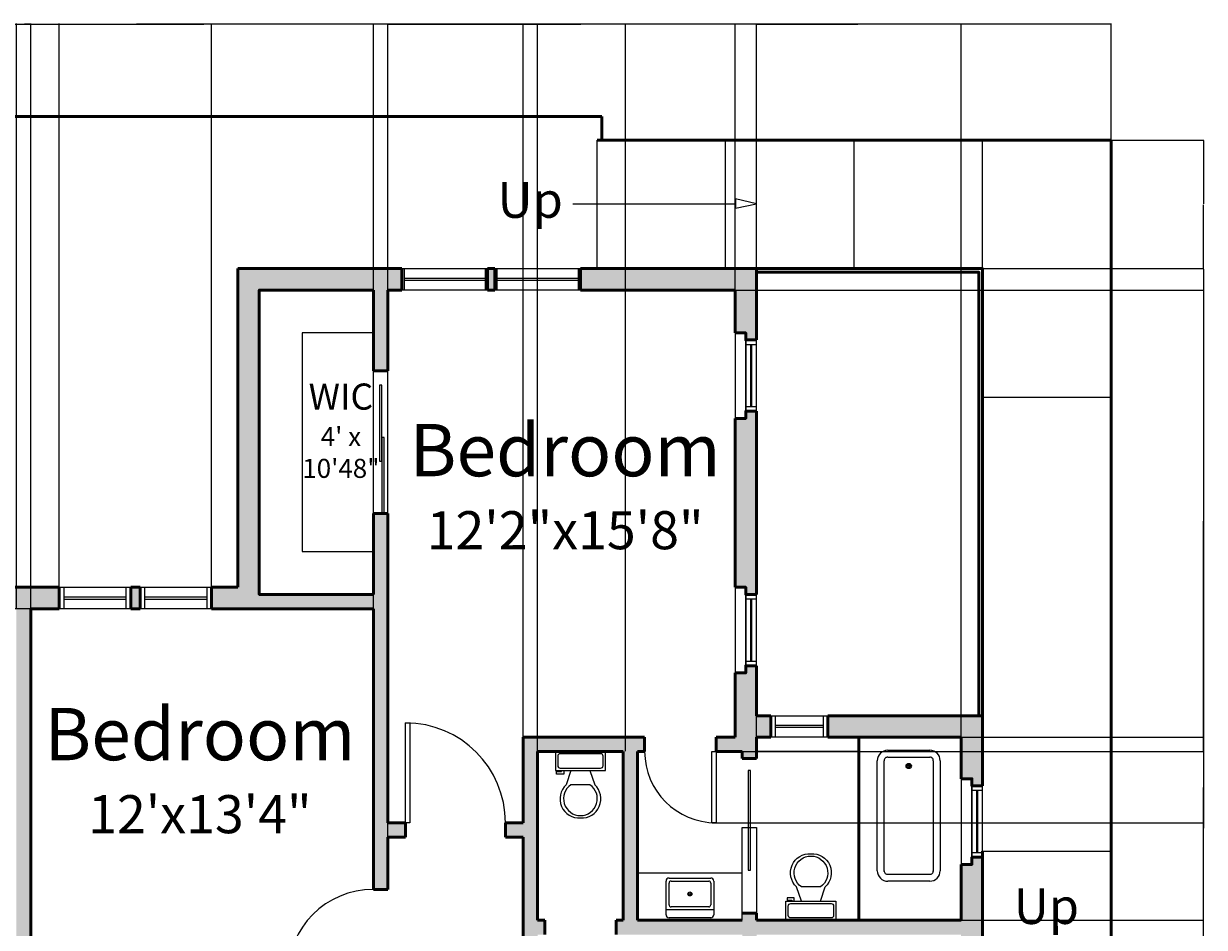
# Model space of a CAD drawing. Units: inches. Extents: x 296 to 2116, y 330 to 1460.
# Tile 9 of 9: x 1620 to 2116, y 1077 to 1457. Entities that reach past the tile are written whole.
import ezdxf

# ---------------------------------------------------------------- set-up
doc = ezdxf.new("R2010")
doc.units = ezdxf.units.IN
for name, color, linetype, lineweight in [('A-ANNO-DIMS', 2, 'Continuous', 18), ('A-ANNO-TEXT', 7, 'Continuous', 18), ('A-AREA-IDEN', 7, 'Continuous', 25), ('A-DOOR', 3, 'Continuous', 25), ('A-FLOR-FIXT', 8, 'Continuous', 18), ('A-FLOR-STRS', 40, 'Continuous', 25), ('A-GLAZ', 4, 'Continuous', 25), ('A-WALL', 7, 'Continuous', 50), ('A-WALL-PATT', 8, 'Continuous', 13)]:
    doc.layers.add(name, color=color, linetype=linetype, lineweight=lineweight)
doc.styles.add('ATTR', font='romans.shx', dxfattribs={"width": 0.8, "height": 1.075})
doc.styles.get("Standard").update_dxf_attribs({"font": 'arial.ttf'})
doc.dimstyles.get("Standard").update_dxf_attribs({"dimtxt": 0.18, "dimasz": 0.18, "dimexe": 0.18, "dimexo": 0.0625, "dimgap": 0.09, "dimtad": 0, "dimtih": 1, "dimtoh": 1, "dimdec": 4, "dimzin": 0, "dimdsep": 46, "dimtxsty": 'Standard', "dimcen": 0.09, "dimadec": 0, "dimazin": 0, "dimtfac": 1, "dimtdec": 4, "dimtofl": 0, "dimtmove": 0, "dimatfit": 3, "dimfxl": 1, "dimtolj": 1, "dimtzin": 0, "dimarcsym": 0})

# ---------------------------------------------------------------- blocks, each defined once
blk = doc.blocks.new('*U19')
for p, q in [((0, 0), (0, -4)), ((36, 0), (36, -4))]:
    blk.add_line(p, q)
blk.add_lwpolyline([(0, 0), (0, 36), (1.75, 36), (1.75, 0)], close=True)
blk.add_arc((0, 0), 36, 0, 90)
blk = doc.blocks.new('*U20')
for p, q in [((0, 0), (0, -4)), ((40, 0), (40, -4))]:
    blk.add_line(p, q)
blk.add_lwpolyline([(0, 0), (0, 40), (1.75, 40), (1.75, 0)], close=True)
blk.add_arc((0, 0), 40, 0, 90)
blk = doc.blocks.new('*U21')
for p, q in [((-30, 0), (-30, 4)), ((0, 0), (0, 4))]:
    blk.add_line(p, q)
blk.add_lwpolyline([(0, 0), (0, -30), (-1.75, -30), (-1.75, 0)], close=True)
blk.add_arc((0, 0), 30, 180, 270)
blk = doc.blocks.new('*U29')
for p, q in [((9.5, -6), (9.5, -2)), ((-10, -8.5), (-8, -8.5)), ((-10, -9.5), (-10, -8.5)), ((-7, -9.5), (-10, -9.5)), ((-8, -8.5), (-8, -8)), ((-7, -8), (-7, -9.5)), ((-4, -8), (-6, -14)), ((4, -8), (6, -14)), ((4, -14), (-4, -14))]:
    blk.add_line(p, q)
blk.add_lwpolyline([(10.5, -8), (10.5, 0), (-10.5, 0), (-10.5, -8)], close=True)
for points in [[(-9.5, -2), (-9.5, -6)], [(8.5, -1), (-8.5, -1)], [(-8.5, -7), (8.5, -7)]]:
    blk.add_lwpolyline(points)
for centre, radius, start, end in [((-8.625, -1.875), 0.8839, 81.8699, 188.1301), ((8.625, -1.875), 0.8839, 351.8699, 98.1301), ((-8.625, -6.125), 0.8839, 171.869898, 278.1301), ((8.625, -6.125), 0.8839, 261.8699, 8.1301), ((-0.4772, -19.9188), 8.0953, 133.01722, 273.38), ((0.0374, -19.8731), 7.127, 124.50543, 269.7), ((-0.0373, -19.8731), 7.127, 270.3, 55.4946), ((0.4773, -19.9188), 8.0953, 266.62, 46.9828)]:
    blk.add_arc(centre, radius, start, end)
blk = doc.blocks.new("24'' Sink Single PV")
blk.add_line((-12.00001, -3.999996), (12, -3.999996))
for points in [[(-10.5, 0), (10.5, 0)], [(-12.00001, -18.499996), (-12.00001, -1.5)], [(-9.5, -5.499996), (9.5, -5.499996)], [(12, -1.5), (12, -18.499996)], [(-10.5, -17.499996), (-10.5, -6.499996)], [(10.5, -6.499996), (10.5, -17.499996)], [(10.5, -19.999996), (-10.5, -19.999996)], [(9.5, -18.499996), (-9.5, -18.499996)]]:
    blk.add_lwpolyline(points)
for radius in [1, 0.5]:
    blk.add_circle((0, -11.999996), radius)
for centre, radius, start, end in [((-10.5, -1.5), 1.5, 90, 180), ((-9.5, -6.499996), 1, 90, 180), ((9.5, -6.499996), 1, 0, 90), ((10.5, -1.5), 1.5, 0, 90), ((-9.5, -17.499996), 1, 180, 270), ((9.5, -17.499996), 1, 270, 0), ((-10.5, -18.499996), 1.5, 180, 270), ((10.5, -18.499996), 1.5, 270, 0)]:
    blk.add_arc(centre, radius, start, end)
at = {"style": 'ATTR', "width": 0.8, "flags": 9}
blk.add_attdef('ESTCODE', (0, 0), '', height=0.0048, dxfattribs=at)
blk = doc.blocks.new('Bath Tub - 26 x 60 in.')
for p, q in [((6, 0), (69, 0)), ((0, -30), (0, -6)), ((75, -6), (75, -30)), ((8, -18), (10, -18)), ((9, -17), (9, -19)), ((69, -36), (6, -36))]:
    blk.add_line(p, q)
for points in [[(4, -30), (4, -6)], [(6, -4), (69.5, -4)], [(71, -30), (71, -6)], [(69.5, -32), (6, -32)]]:
    blk.add_lwpolyline(points)
for radius in [1.5, 1]:
    blk.add_circle((9, -18), radius)
for centre, radius, start, end in [((6, -6), 6, 90, 180), ((69, -6), 6, 0, 90), ((5.75, -5.75), 1.77, 81.8699, 188.1301), ((69.25, -5.75), 1.77, 351.8699, 98.1301), ((6, -30), 6, 180, 270), ((5.75, -30.25), 1.77, 171.8699, 278.1301), ((69.25, -30.25), 1.77, 261.8699, 8.1301), ((69, -30), 6, 270, 0)]:
    blk.add_arc(centre, radius, start, end)
blk = doc.blocks.new('*D67')
at = {"layer": 'A-ANNO-DIMS', "color": 0, "lineweight": -2, "transparency": 16777216}
for p, q in [((1315.18, 1418.02), (1315.18, 1456.98)), ((1315.36, 1456.8), (1695.9, 1456.8)), ((2077, 1456.8), (1696.47, 1456.8)), ((2077.18, 1408.02), (2077.18, 1456.98))]:
    blk.add_line(p, q, dxfattribs=at)
at = {"layer": 'A-ANNO-DIMS', "color": 0, "transparency": 16777216}
for points in [[(1315.36, 1456.83), (1315.36, 1456.77), (1315.18, 1456.8)], [(2077, 1456.83), (2077, 1456.77), (2077.18, 1456.8)]]:
    blk.add_solid(points, dxfattribs=at)
at = {"layer": 'Defpoints', "color": 0, "transparency": 16777216}
for p in [(2077.18, 1456.8), (1315.18, 1417.95), (2077.18, 1407.95)]:
    blk.add_point(p, dxfattribs=at)
at = {"layer": 'A-ANNO-DIMS', "color": 0, "transparency": 16777216, "insert": (1696.18, 1456.8), "char_height": 0.18, "attachment_point": 5}
blk.add_mtext('\\A1;762', dxfattribs=at)
blk = doc.blocks.new('*D74')
at = {"layer": 'A-ANNO-DIMS', "color": 0, "lineweight": -2, "transparency": 16777216}
for p, q in [((2023.25, 1353.95), (2116.21, 1353.95)), ((2116.03, 1353.77), (2116.03, 1129.14)), ((2116.03, 904.13), (2116.03, 1128.77)), ((2023.25, 903.95), (2116.21, 903.95))]:
    blk.add_line(p, q, dxfattribs=at)
at = {"layer": 'A-ANNO-DIMS', "color": 0, "transparency": 16777216}
for points in [[(2116, 1353.77), (2116.06, 1353.77), (2116.03, 1353.95)], [(2116, 904.13), (2116.06, 904.13), (2116.03, 903.95)]]:
    blk.add_solid(points, dxfattribs=at)
at = {"layer": 'Defpoints', "color": 0, "transparency": 16777216}
for p in [(2023.18, 1353.95), (2116.03, 1353.95), (2023.18, 903.95)]:
    blk.add_point(p, dxfattribs=at)
at = {"layer": 'A-ANNO-DIMS', "color": 0, "transparency": 16777216, "insert": (2116.03, 1128.95), "char_height": 0.18, "attachment_point": 5}
blk.add_mtext('\\A1;450', dxfattribs=at)
blk = doc.blocks.new('*D75')
at = {"layer": 'A-ANNO-DIMS', "color": 0, "lineweight": -2, "transparency": 16777216}
for p, q in [((2077.25, 1407.95), (2116.21, 1407.95)), ((2116.03, 1407.77), (2116.03, 1381.14)), ((2116.03, 1354.13), (2116.03, 1380.77)), ((2023.25, 1353.95), (2116.21, 1353.95))]:
    blk.add_line(p, q, dxfattribs=at)
at = {"layer": 'A-ANNO-DIMS', "color": 0, "transparency": 16777216}
for points in [[(2116, 1407.77), (2116.06, 1407.77), (2116.03, 1407.95)], [(2116, 1354.13), (2116.06, 1354.13), (2116.03, 1353.95)]]:
    blk.add_solid(points, dxfattribs=at)
at = {"layer": 'Defpoints', "color": 0, "transparency": 16777216}
for p in [(2077.18, 1407.95), (2116.03, 1407.95), (2023.18, 1353.95)]:
    blk.add_point(p, dxfattribs=at)
at = {"layer": 'A-ANNO-DIMS', "color": 0, "transparency": 16777216, "insert": (2116.03, 1380.95), "char_height": 0.18, "attachment_point": 5}
blk.add_mtext('\\A1;54', dxfattribs=at)
blk = doc.blocks.new('*D108')
at = {"layer": 'A-ANNO-DIMS', "color": 0, "lineweight": -2, "transparency": 16777216}
for p, q in [((1617.18, 1211.02), (1617.18, 1456.98)), ((1617.36, 1456.8), (1619.86, 1456.8)), ((1623, 1456.8), (1620.51, 1456.8)), ((1623.18, 1211.02), (1623.18, 1456.98))]:
    blk.add_line(p, q, dxfattribs=at)
at = {"layer": 'A-ANNO-DIMS', "color": 0, "transparency": 16777216}
for points in [[(1617.36, 1456.83), (1617.36, 1456.77), (1617.18, 1456.8)], [(1623, 1456.83), (1623, 1456.77), (1623.18, 1456.8)]]:
    blk.add_solid(points, dxfattribs=at)
at = {"layer": 'Defpoints', "color": 0, "transparency": 16777216}
for p in [(1623.18, 1456.8), (1617.18, 1210.95), (1623.18, 1210.95)]:
    blk.add_point(p, dxfattribs=at)
at = {"layer": 'A-ANNO-DIMS', "color": 0, "transparency": 16777216, "insert": (1620.18, 1456.8), "char_height": 0.18, "attachment_point": 5}
blk.add_mtext('\\A1;6.00', dxfattribs=at)
blk = doc.blocks.new('*D109')
at = {"layer": 'A-ANNO-DIMS', "color": 0, "lineweight": -2, "transparency": 16777216}
for p, q in [((1623.18, 1211.02), (1623.18, 1456.98)), ((1623.36, 1456.8), (1694.73, 1456.8)), ((1767, 1456.8), (1695.64, 1456.8)), ((1767.18, 1211.02), (1767.18, 1456.98))]:
    blk.add_line(p, q, dxfattribs=at)
at = {"layer": 'A-ANNO-DIMS', "color": 0, "transparency": 16777216}
for points in [[(1623.36, 1456.83), (1623.36, 1456.77), (1623.18, 1456.8)], [(1767, 1456.83), (1767, 1456.77), (1767.18, 1456.8)]]:
    blk.add_solid(points, dxfattribs=at)
at = {"layer": 'Defpoints', "color": 0, "transparency": 16777216}
for p in [(1767.18, 1456.8), (1623.18, 1210.95), (1767.18, 1210.95)]:
    blk.add_point(p, dxfattribs=at)
at = {"layer": 'A-ANNO-DIMS', "color": 0, "transparency": 16777216, "insert": (1695.18, 1456.8), "char_height": 0.18, "attachment_point": 5}
blk.add_mtext('\\A1;144.00', dxfattribs=at)
blk = doc.blocks.new('*D110')
at = {"layer": 'A-ANNO-DIMS', "color": 0, "lineweight": -2, "transparency": 16777216}
for p, q in [((1773.18, 1345.02), (1773.18, 1456.98)), ((1773.36, 1456.8), (1845.73, 1456.8)), ((1919, 1456.8), (1846.64, 1456.8)), ((1919.18, 1345.02), (1919.18, 1456.98))]:
    blk.add_line(p, q, dxfattribs=at)
at = {"layer": 'A-ANNO-DIMS', "color": 0, "transparency": 16777216}
for points in [[(1773.36, 1456.83), (1773.36, 1456.77), (1773.18, 1456.8)], [(1919, 1456.83), (1919, 1456.77), (1919.18, 1456.8)]]:
    blk.add_solid(points, dxfattribs=at)
at = {"layer": 'Defpoints', "color": 0, "transparency": 16777216}
for p in [(1919.18, 1456.8), (1773.18, 1344.95), (1919.18, 1344.95)]:
    blk.add_point(p, dxfattribs=at)
at = {"layer": 'A-ANNO-DIMS', "color": 0, "transparency": 16777216, "insert": (1846.18, 1456.8), "char_height": 0.18, "attachment_point": 5}
blk.add_mtext('\\A1;146.00', dxfattribs=at)
blk = doc.blocks.new('*D118')
at = {"layer": 'A-ANNO-DIMS', "color": 0, "lineweight": -2, "transparency": 16777216}
for p, q in [((1623.12, 1210.95), (1276.15, 1210.95)), ((1276.33, 1210.77), (1276.33, 1131.14)), ((1276.33, 1051.13), (1276.33, 1130.77)), ((1623.12, 1050.95), (1276.15, 1050.95))]:
    blk.add_line(p, q, dxfattribs=at)
at = {"layer": 'A-ANNO-DIMS', "color": 0, "transparency": 16777216}
for points in [[(1276.3, 1210.77), (1276.36, 1210.77), (1276.33, 1210.95)], [(1276.3, 1051.13), (1276.36, 1051.13), (1276.33, 1050.95)]]:
    blk.add_solid(points, dxfattribs=at)
at = {"layer": 'Defpoints', "color": 0, "transparency": 16777216}
for p in [(1276.33, 1210.95), (1623.18, 1210.95), (1623.18, 1050.95)]:
    blk.add_point(p, dxfattribs=at)
at = {"layer": 'A-ANNO-DIMS', "color": 0, "transparency": 16777216, "insert": (1276.33, 1130.95), "char_height": 0.18, "attachment_point": 5}
blk.add_mtext('\\A1;160.00', dxfattribs=at)
blk = doc.blocks.new('*D119')
at = {"layer": 'A-ANNO-DIMS', "color": 0, "lineweight": -2, "transparency": 16777216}
for p, q in [((1773.183215, 1093.016598), (1773.183215, 1456.984098)), ((1773.363215, 1456.804098), (1801.289818, 1456.804098)), ((1830.003215, 1456.804098), (1802.076612, 1456.804098)), ((1830.183215, 1157.016598), (1830.183215, 1456.984098))]:
    blk.add_line(p, q, dxfattribs=at)
at = {"layer": 'A-ANNO-DIMS', "color": 0, "transparency": 16777216}
for points in [[(1773.363215, 1456.834098), (1773.363215, 1456.774098), (1773.183215, 1456.804098)], [(1830.003215, 1456.834098), (1830.003215, 1456.774098), (1830.183215, 1456.804098)]]:
    blk.add_solid(points, dxfattribs=at)
at = {"layer": 'Defpoints', "color": 0, "transparency": 16777216}
for p in [(1830.183215, 1456.804098), (1830.183215, 1156.954098), (1773.183215, 1092.954098)]:
    blk.add_point(p, dxfattribs=at)
at = {"layer": 'A-ANNO-DIMS', "color": 0, "transparency": 16777216, "insert": (1801.683215, 1456.804098), "char_height": 0.18, "attachment_point": 5}
blk.add_mtext('\\A1;57.00', dxfattribs=at)
blk = doc.blocks.new('*D120')
at = {"layer": 'A-ANNO-DIMS', "color": 0, "lineweight": -2, "transparency": 16777216}
for p, q in [((1836.18, 1151.02), (1836.18, 1456.98)), ((1836.36, 1456.8), (1854.29, 1456.8)), ((1873, 1456.8), (1855.08, 1456.8)), ((1873.18, 1151.02), (1873.18, 1456.98))]:
    blk.add_line(p, q, dxfattribs=at)
at = {"layer": 'A-ANNO-DIMS', "color": 0, "transparency": 16777216}
for points in [[(1836.36, 1456.83), (1836.36, 1456.77), (1836.18, 1456.8)], [(1873, 1456.83), (1873, 1456.77), (1873.18, 1456.8)]]:
    blk.add_solid(points, dxfattribs=at)
at = {"layer": 'Defpoints', "color": 0, "transparency": 16777216}
for p in [(1873.18, 1456.8), (1836.18, 1150.95), (1873.18, 1150.95)]:
    blk.add_point(p, dxfattribs=at)
at = {"layer": 'A-ANNO-DIMS', "color": 0, "transparency": 16777216, "insert": (1854.68, 1456.8), "char_height": 0.18, "attachment_point": 5}
blk.add_mtext('\\A1;37.00', dxfattribs=at)
blk = doc.blocks.new('*D121')
at = {"layer": 'A-ANNO-DIMS', "color": 0, "lineweight": -2, "transparency": 16777216}
for p, q in [((1928.18, 1151.02), (1928.18, 1456.98)), ((1928.36, 1456.8), (1970.79, 1456.8)), ((2014, 1456.8), (1971.58, 1456.8)), ((2014.18, 1157.02), (2014.18, 1456.98))]:
    blk.add_line(p, q, dxfattribs=at)
at = {"layer": 'A-ANNO-DIMS', "color": 0, "transparency": 16777216}
for points in [[(1928.36, 1456.83), (1928.36, 1456.77), (1928.18, 1456.8)], [(2014, 1456.83), (2014, 1456.77), (2014.18, 1456.8)]]:
    blk.add_solid(points, dxfattribs=at)
at = {"layer": 'Defpoints', "color": 0, "transparency": 16777216}
for p in [(2014.18, 1456.8), (2014.18, 1156.95), (1928.18, 1150.95)]:
    blk.add_point(p, dxfattribs=at)
at = {"layer": 'A-ANNO-DIMS', "color": 0, "transparency": 16777216, "insert": (1971.18, 1456.8), "char_height": 0.18, "attachment_point": 5}
blk.add_mtext('\\A1;86.00', dxfattribs=at)
blk = doc.blocks.new('*D124')
at = {"layer": 'A-ANNO-DIMS', "color": 0, "lineweight": -2, "transparency": 16777216}
for p, q in [((2014.25, 1156.95), (2116.21, 1156.95)), ((2116.03, 1156.77), (2116.03, 1118.64)), ((2116.03, 1080.13), (2116.03, 1118.27)), ((2014.25, 1079.95), (2116.21, 1079.95))]:
    blk.add_line(p, q, dxfattribs=at)
at = {"layer": 'A-ANNO-DIMS', "color": 0, "transparency": 16777216}
for points in [[(2116, 1156.77), (2116.06, 1156.77), (2116.03, 1156.95)], [(2116, 1080.13), (2116.06, 1080.13), (2116.03, 1079.95)]]:
    blk.add_solid(points, dxfattribs=at)
at = {"layer": 'Defpoints', "color": 0, "transparency": 16777216}
for p in [(2014.18, 1156.95), (2116.03, 1156.95), (2014.18, 1079.95)]:
    blk.add_point(p, dxfattribs=at)
at = {"layer": 'A-ANNO-DIMS', "color": 0, "transparency": 16777216, "insert": (2116.03, 1118.45), "char_height": 0.18, "attachment_point": 5}
blk.add_mtext('\\A1;77.00', dxfattribs=at)
blk = doc.blocks.new('*D125')
at = {"layer": 'A-ANNO-DIMS', "color": 0, "lineweight": -2, "transparency": 16777216}
for p, q in [((1919.25, 1344.95), (2116.21, 1344.95)), ((2116.03, 1344.77), (2116.03, 1248.14)), ((2116.03, 1151.13), (2116.03, 1247.77)), ((1922.25, 1150.95), (2116.21, 1150.95))]:
    blk.add_line(p, q, dxfattribs=at)
at = {"layer": 'A-ANNO-DIMS', "color": 0, "transparency": 16777216}
for points in [[(2116, 1344.77), (2116.06, 1344.77), (2116.03, 1344.95)], [(2116, 1151.13), (2116.06, 1151.13), (2116.03, 1150.95)]]:
    blk.add_solid(points, dxfattribs=at)
at = {"layer": 'Defpoints', "color": 0, "transparency": 16777216}
for p in [(1919.18, 1344.95), (2116.03, 1344.95), (1922.18, 1150.95)]:
    blk.add_point(p, dxfattribs=at)
at = {"layer": 'A-ANNO-DIMS', "color": 0, "transparency": 16777216, "insert": (2116.03, 1247.95), "char_height": 0.18, "attachment_point": 5}
blk.add_mtext('\\A1;194.00', dxfattribs=at)
blk = doc.blocks.new('*D128')
at = {"layer": 'A-ANNO-DIMS', "color": 0, "lineweight": -2, "transparency": 16777216}
for p, q in [((1909.5, 1150.95), (2116.21, 1150.95)), ((2116.03, 1150.77), (2116.03, 1136.14)), ((2116.03, 1121.13), (2116.03, 1135.77)), ((1909.5, 1120.95), (2116.21, 1120.95))]:
    blk.add_line(p, q, dxfattribs=at)
at = {"layer": 'A-ANNO-DIMS', "color": 0, "transparency": 16777216}
for points in [[(2116, 1150.77), (2116.06, 1150.77), (2116.03, 1150.95)], [(2116, 1121.13), (2116.06, 1121.13), (2116.03, 1120.95)]]:
    blk.add_solid(points, dxfattribs=at)
at = {"layer": 'Defpoints', "color": 0, "transparency": 16777216}
for p in [(1909.43, 1150.95), (1909.43, 1120.95), (2116.03, 1120.95)]:
    blk.add_point(p, dxfattribs=at)
at = {"layer": 'A-ANNO-DIMS', "color": 0, "transparency": 16777216, "insert": (2116.03, 1135.95), "char_height": 0.18, "attachment_point": 5}
blk.add_mtext('\\A1;30.00', dxfattribs=at)
blk = doc.blocks.new('*D131')
at = {"layer": 'A-ANNO-DIMS', "color": 0, "lineweight": -2, "transparency": 16777216}
for p, q in [((1635.18, 1220.02), (1635.18, 1456.98)), ((1635.36, 1456.8), (1666.79, 1456.8)), ((1699, 1456.8), (1667.58, 1456.8)), ((1699.18, 1220.02), (1699.18, 1456.98))]:
    blk.add_line(p, q, dxfattribs=at)
at = {"layer": 'A-ANNO-DIMS', "color": 0, "transparency": 16777216}
for points in [[(1635.36, 1456.83), (1635.36, 1456.77), (1635.18, 1456.8)], [(1699, 1456.83), (1699, 1456.77), (1699.18, 1456.8)]]:
    blk.add_solid(points, dxfattribs=at)
at = {"layer": 'Defpoints', "color": 0, "transparency": 16777216}
for p in [(1699.18, 1456.8), (1635.18, 1219.95), (1699.18, 1219.95)]:
    blk.add_point(p, dxfattribs=at)
at = {"layer": 'A-ANNO-DIMS', "color": 0, "transparency": 16777216, "insert": (1667.18, 1456.8), "char_height": 0.18, "attachment_point": 5}
blk.add_mtext('\\A1;64.00', dxfattribs=at)

msp = doc.modelspace()

# ---------------------------------------------------------------- hatches: boundary and pattern name
at = {"layer": 'A-WALL-PATT'}
h = msp.add_hatch(color=256, dxfattribs=at)
h.dxf.hatch_style = 1
h.paths.add_polyline_path([(1321.1832, 1353.9541), (1315.1832, 1353.9541), (1315.1832, 1347.9541), (1321.1832, 1347.9541)])
h.paths.add_polyline_path([(1496.1832, 1353.9541), (1490.1832, 1353.9541), (1490.1832, 1347.9541), (1496.1832, 1347.9541)])
h.paths.add_polyline_path([(1396.1832, 1189.9541), (1392.1832, 1189.9541), (1392.1832, 1180.9541), (1396.1832, 1180.9541)])
h.paths.add_polyline_path([(1436.1832, 1189.9541), (1432.1832, 1189.9541), (1432.1832, 1180.9541), (1436.1832, 1180.9541), (1436.1832, 1184.9541)])
h.paths.add_polyline_path([(1356.1832, 1189.9541), (1318.1832, 1189.9541), (1318.1832, 1138.9541), (1322.6832, 1138.9541), (1322.6832, 1144.9541), (1327.1832, 1144.9541), (1327.1832, 1180.9541), (1356.1832, 1180.9541)])
h.paths.add_polyline_path([(1499.1832, 1210.9541), (1523.1832, 1210.9541), (1523.1832, 1219.9541), (1490.1832, 1219.9541), (1490.1832, 1189.9541), (1472.1832, 1189.9541), (1472.1832, 1180.9541), (1499.1832, 1180.9541)])
h.paths.add_polyline_path([(1635.1832, 1219.9541), (1599.1832, 1219.9541), (1599.1832, 1210.9541), (1617.1832, 1210.9541), (1617.1832, 1050.9541), (1581.1832, 1050.9541), (1581.1832, 1041.9541), (1587.1832, 1041.9541), (1587.1832, 1044.9541), (1617.1832, 1044.9541), (1617.1832, 978.9541), (1587.1832, 978.9541), (1587.1832, 981.9541), (1581.1832, 981.9541), (1581.1832, 966.9541), (1587.1832, 966.9541), (1587.1832, 972.9541), (1773.1832, 972.9541), (1773.1832, 981.9541), (1767.1832, 981.9541), (1767.1832, 978.9541), (1733.1832, 978.9541), (1733.1832, 1044.9541), (1767.1832, 1044.9541), (1767.1832, 1041.9541), (1773.1832, 1041.9541), (1773.1832, 1056.9541), (1767.1832, 1056.9541), (1767.1832, 1050.9541), (1705.1832, 1050.9541), (1705.1832, 1044.9541), (1727.1832, 1044.9541), (1727.1832, 978.9541), (1623.1832, 978.9541), (1623.1832, 1044.9541), (1645.1832, 1044.9541), (1645.1832, 1050.9541), (1623.1832, 1050.9541), (1623.1832, 1210.9541), (1635.1832, 1210.9541)])
h.paths.add_polyline_path([(1773.1832, 1250.9541), (1767.1832, 1250.9541), (1767.1832, 1216.9541), (1719.1832, 1216.9541), (1719.1832, 1344.9541), (1767.1832, 1344.9541), (1767.1832, 1310.9541), (1773.1832, 1310.9541), (1773.1832, 1344.9541), (1779.1832, 1344.9541), (1779.1832, 1353.9541), (1710.1832, 1353.9541), (1710.1832, 1219.9541), (1699.1832, 1219.9541), (1699.1832, 1210.9541), (1767.1832, 1210.9541), (1767.1832, 1092.9541), (1773.1832, 1092.9541), (1773.1832, 1114.9541), (1780.6832, 1114.9541), (1780.6832, 1120.9541), (1773.1832, 1120.9541)])
h.paths.add_polyline_path([(1360.1832, 899.9541), (1327.1832, 899.9541), (1327.1832, 918.4541), (1322.6832, 918.4541), (1322.6832, 921.4541), (1318.1832, 921.4541), (1318.1832, 890.9541), (1351.1832, 890.9541), (1351.1832, 817.9991), (1590.1832, 817.9991), (1590.1832, 903.9541), (1614.1832, 903.9541), (1614.1832, 912.9541), (1587.1832, 912.9541), (1587.1832, 918.9541), (1581.1832, 918.9541), (1581.1832, 880.9991), (1420.1332, 880.9991), (1420.1332, 918.9541), (1415.9332, 918.9541), (1414.1332, 918.9541), (1414.1332, 874.9991), (1581.1832, 874.9991), (1581.1832, 826.9991), (1360.1832, 826.9991)])
h.paths.add_polyline_path([(1327.1832, 1056.9541), (1322.6832, 1056.9541), (1322.6832, 1062.9541), (1318.1832, 1062.9541), (1318.1832, 951.4541), (1322.6832, 951.4541), (1322.6832, 954.4541), (1327.1832, 954.4541), (1327.1832, 972.9541), (1414.1332, 972.9541), (1414.1332, 960.9541), (1420.1332, 960.9541), (1420.1332, 978.9541), (1327.1832, 978.9541)])
h.paths.add_polyline_path([(2023.1832, 1106.4482), (2018.6832, 1106.4482), (2018.6832, 1103.4482), (2014.1832, 1103.4482), (2014.1832, 1079.9541), (1928.1832, 1079.9541), (1928.1832, 1082.9541), (1922.1832, 1082.9541), (1922.1832, 1079.9541), (1878.1832, 1079.9541), (1878.1832, 1150.9541), (1881.1832, 1150.9541), (1881.1832, 1154.9541), (1881.1832, 1156.9541), (1830.1832, 1156.9541), (1830.1832, 1120.9541), (1822.6832, 1120.9541), (1822.6832, 1116.7541), (1822.6832, 1114.9541), (1830.1832, 1114.9541), (1830.1832, 1067.9541), (1834.1832, 1067.9541), (1836.1832, 1067.9541), (1836.1832, 1073.9541), (1839.1832, 1073.9541), (1839.1832, 1079.9541), (1836.1832, 1079.9541), (1836.1832, 1150.9541), (1872.1832, 1150.9541), (1872.1832, 1079.9541), (1869.1832, 1079.9541), (1869.1832, 1073.9541), (1905.1832, 1073.9541), (1922.1832, 1073.9541), (1922.1832, 1067.9541), (1926.1832, 1067.9541), (1928.1832, 1067.9541), (1928.1832, 1073.9541), (2014.1832, 1073.9541), (2014.1832, 1002.9541), (1970.1832, 1002.9541), (1928.1832, 1002.9541), (1928.1832, 1031.9541), (1922.1832, 1031.9541), (1922.1832, 1002.9541), (1836.1832, 1002.9541), (1836.1832, 1031.9541), (1834.1832, 1031.9541), (1830.1832, 1031.9541), (1830.1832, 978.9541), (1836.1832, 978.9541), (1836.1832, 996.9541), (2014.1832, 996.9541), (2014.1832, 912.9541), (1836.1832, 912.9541), (1836.1832, 942.9541), (1832.1832, 942.9541), (1830.1832, 942.9541), (1830.1832, 912.9541), (1656.1832, 912.9541), (1656.1832, 908.7541), (1656.1832, 903.9541), (2023.1832, 903.9541)])
h.paths.add_polyline_path([(2023.1832, 1165.9541), (1958.1832, 1165.9541), (1958.1832, 1156.9541), (2014.1832, 1156.9541), (2014.1832, 1139.4482), (2018.6832, 1139.4482), (2018.6832, 1136.4482), (2023.1832, 1136.4482), (2023.1832, 1159.9541)])
h.paths.add_polyline_path([(1934.1832, 1165.9541), (1928.1832, 1165.9541), (1928.1832, 1186.9541), (1923.6832, 1186.9541), (1923.6832, 1183.9541), (1919.1832, 1183.9541), (1919.1832, 1156.9541), (1911.1832, 1156.9541), (1911.1832, 1150.9541), (1922.1832, 1150.9541), (1922.1832, 1147.9541), (1928.1832, 1147.9541), (1928.1832, 1156.9541), (1934.1832, 1156.9541)])
h.paths.add_polyline_path([(1928.1832, 1293.9541), (1923.6832, 1293.9541), (1923.6832, 1290.9541), (1919.1832, 1290.9541), (1919.1832, 1219.9541), (1923.6832, 1219.9541), (1923.6832, 1216.9541), (1928.1832, 1216.9541)])
h.paths.add_polyline_path([(1928.1832, 1353.9541), (1854.1832, 1353.9541), (1854.1832, 1344.9541), (1919.1832, 1344.9541), (1919.1832, 1326.9541), (1923.6832, 1326.9541), (1923.6832, 1323.9541), (1928.1832, 1323.9541)])
h.paths.add_polyline_path([(1818.1832, 1353.9541), (1815.1832, 1353.9541), (1815.1832, 1344.9541), (1818.1832, 1344.9541)])
h.paths.add_polyline_path([(1563.1832, 1219.9541), (1559.1832, 1219.9541), (1559.1832, 1210.9541), (1563.1832, 1210.9541)])
h.paths.add_polyline_path([(1669.1832, 1219.9541), (1665.1832, 1219.9541), (1665.1832, 1210.9541), (1669.1832, 1210.9541)])
h.paths.add_polyline_path([(1322.6832, 1102.9541), (1318.1832, 1102.9541), (1318.1832, 1098.9541), (1322.6832, 1098.9541)])

# ---------------------------------------------------------------- linework, layer by layer
at = {"layer": 'A-DOOR'}
for points in [[(1769.6832, 1272.9541), (1770.6832, 1272.9541), (1770.6832, 1304.9541), (1769.6832, 1304.9541)], [(1770.6832, 1250.9541), (1771.6832, 1250.9541), (1771.6832, 1282.9541), (1770.6832, 1282.9541)], [(1925.6832, 1100.9541), (1925.6832, 1142.9541), (1924.6832, 1142.9541), (1924.6832, 1100.9541)], [(1922.1832, 1082.9541), (1922.1832, 1118.9541), (1928.1832, 1118.9541), (1928.1832, 1082.9541)]]:
    msp.add_lwpolyline(points, close=True, dxfattribs=at)
at = {"layer": 'A-FLOR-FIXT'}
for p, q in [((1971.1832, 1150.9541), (1928.1832, 1150.9541)), ((1878.1832, 1099.9541), (1922.1832, 1099.9541)), ((1922.1832, 1079.9541), (1922.1832, 1099.9541))]:
    msp.add_line(p, q, dxfattribs=at)
msp.add_lwpolyline([(1767.1832, 1326.9541), (1737.1832, 1326.9541), (1737.1832, 1234.9541), (1767.1832, 1234.9541)], dxfattribs=at)
at = {"layer": 'A-FLOR-STRS'}
for p, q in [((1861.1832, 1353.9541), (1861.1832, 1407.9541)), ((1915.1832, 1353.9541), (1915.1832, 1407.9541)), ((1969.1832, 1353.9541), (1969.1832, 1407.9541)), ((2023.1832, 1353.9541), (2023.1832, 1407.9541)), ((2023.1832, 1353.9541), (2077.1832, 1353.9541)), ((2023.1832, 1299.9541), (2077.1832, 1299.9541)), ((2023.1832, 1156.9541), (2077.1832, 1156.9541)), ((2023.1832, 1108.9541), (2077.1832, 1108.9541))]:
    msp.add_line(p, q, dxfattribs=at)
msp.add_lwpolyline([(1850.9688, 1381.1525), (1919.3093, 1381.1525)], dxfattribs=at)
msp.add_lwpolyline([(1928.1772, 1381.1525), (1919.3093, 1383.2975), (1919.3093, 1379.4043)], close=True, dxfattribs=at)
at = {"layer": 'A-GLAZ'}
for p, q in [((1780.1832, 1344.9541), (1780.1832, 1353.9541)), ((1780.1832, 1349.9541), (1814.1832, 1349.9541)), ((1814.1832, 1353.9541), (1814.1832, 1344.9541)), ((1819.1832, 1344.9541), (1819.1832, 1353.9541)), ((1819.1832, 1349.9541), (1853.1832, 1349.9541)), ((1853.1832, 1353.9541), (1853.1832, 1344.9541)), ((1814.1832, 1348.9541), (1780.1832, 1348.9541)), ((1853.1832, 1348.9541), (1819.1832, 1348.9541)), ((1928.1832, 1321.9541), (1923.6832, 1321.9541)), ((1925.6832, 1321.9541), (1925.6832, 1295.9541)), ((1926.1832, 1295.9541), (1926.1832, 1321.9541)), ((1923.6832, 1295.9541), (1928.1832, 1295.9541)), ((1637.1832, 1215.9541), (1663.1832, 1215.9541)), ((1671.1832, 1215.9541), (1697.1832, 1215.9541)), ((1637.1832, 1214.9541), (1663.1832, 1214.9541)), ((1671.1832, 1214.9541), (1697.1832, 1214.9541)), ((1928.1832, 1214.9541), (1923.6832, 1214.9541)), ((1925.6832, 1214.9541), (1925.6832, 1188.9541)), ((1926.1832, 1188.9541), (1926.1832, 1214.9541)), ((1923.6832, 1188.9541), (1928.1832, 1188.9541)), ((1936.1832, 1156.9541), (1936.1832, 1165.9541)), ((1936.1832, 1161.9541), (1956.1832, 1161.9541)), ((1956.1832, 1165.9541), (1956.1832, 1156.9541)), ((1956.1832, 1160.9541), (1936.1832, 1160.9541)), ((2023.1832, 1134.4482), (2018.6832, 1134.4482)), ((2020.6832, 1134.4482), (2020.6832, 1108.4482)), ((2021.1832, 1108.4482), (2021.1832, 1134.4482)), ((2018.6832, 1108.4482), (2023.1832, 1108.4482))]:
    msp.add_line(p, q, dxfattribs=at)
for points in [[(1815.1832, 1353.9541), (1815.1832, 1344.9541), (1779.1832, 1344.9541), (1779.1832, 1353.9541)], [(1854.1832, 1353.9541), (1854.1832, 1344.9541), (1818.1832, 1344.9541), (1818.1832, 1353.9541)], [(1919.1832, 1290.9541), (1923.6832, 1290.9541), (1923.6832, 1326.9541), (1919.1832, 1326.9541)], [(1928.1832, 1293.9541), (1928.1832, 1323.9541), (1923.6832, 1323.9541), (1923.6832, 1293.9541)], [(1635.1832, 1219.9541), (1665.1832, 1219.9541), (1665.1832, 1210.9541), (1635.1832, 1210.9541)], [(1669.1832, 1219.9541), (1699.1832, 1219.9541), (1699.1832, 1210.9541), (1669.1832, 1210.9541)], [(1919.1832, 1183.9541), (1923.6832, 1183.9541), (1923.6832, 1219.9541), (1919.1832, 1219.9541)], [(1928.1832, 1186.9541), (1928.1832, 1216.9541), (1923.6832, 1216.9541), (1923.6832, 1186.9541)], [(1958.1832, 1156.9541), (1934.1832, 1156.9541), (1934.1832, 1165.9541), (1958.1832, 1165.9541)], [(2014.1832, 1103.4482), (2018.6832, 1103.4482), (2018.6832, 1139.4482), (2014.1832, 1139.4482)], [(2023.1832, 1106.4482), (2023.1832, 1136.4482), (2018.6832, 1136.4482), (2018.6832, 1106.4482)]]:
    msp.add_lwpolyline(points, close=True, dxfattribs=at)
for points in [[(1637.1832, 1210.9541), (1637.1832, 1219.9541)], [(1663.1832, 1219.9541), (1663.1832, 1210.9541)], [(1671.1832, 1210.9541), (1671.1832, 1219.9541)], [(1697.1832, 1219.9541), (1697.1832, 1210.9541)]]:
    msp.add_lwpolyline(points, dxfattribs=at)
at = {"layer": 'A-WALL'}
for p, q in [((1315.1832, 1417.9541), (1863.1832, 1417.9541)), ((1863.1832, 1417.9541), (1863.1832, 1407.9541)), ((1861.1832, 1407.9541), (2077.1832, 1407.9541)), ((2077.1832, 1407.9541), (2077.1832, 961.9541)), ((1710.1832, 1353.9541), (1779.1832, 1353.9541)), ((1710.1832, 1219.9541), (1710.1832, 1353.9541)), ((1779.1832, 1344.9541), (1779.1832, 1353.9541)), ((1815.1832, 1344.9541), (1815.1832, 1353.9541)), ((1815.1832, 1353.9541), (1818.1832, 1353.9541)), ((1818.1832, 1344.9541), (1818.1832, 1353.9541)), ((1854.1832, 1344.9541), (1854.1832, 1353.9541)), ((1767.1832, 1310.9541), (1767.1832, 1344.9541)), ((1773.1832, 1344.9541), (1779.1832, 1344.9541)), ((1773.1832, 1310.9541), (1773.1832, 1344.9541)), ((1815.1832, 1344.9541), (1818.1832, 1344.9541)), ((1854.1832, 1344.9541), (1919.1832, 1344.9541)), ((1919.1832, 1344.9541), (1919.1832, 1326.9541)), ((1767.1832, 1310.9541), (1773.1832, 1310.9541)), ((1919.1832, 1290.9541), (1919.1832, 1219.9541)), ((1767.1832, 1216.9541), (1767.1832, 1250.9541)), ((1767.1832, 1250.9541), (1773.1832, 1250.9541)), ((1773.1832, 1120.9541), (1773.1832, 1250.9541)), ((1599.1832, 1219.9541), (1635.1832, 1219.9541)), ((1635.1832, 1210.9541), (1635.1832, 1219.9541)), ((1665.1832, 1210.9541), (1665.1832, 1219.9541)), ((1665.1832, 1219.9541), (1669.1832, 1219.9541)), ((1669.1832, 1210.9541), (1669.1832, 1219.9541)), ((1699.1832, 1210.9541), (1699.1832, 1219.9541)), ((1699.1832, 1219.9541), (1710.1832, 1219.9541)), ((1623.1832, 1210.9541), (1635.1832, 1210.9541)), ((1623.1832, 1210.9541), (1623.1832, 1050.9541)), ((1665.1832, 1210.9541), (1669.1832, 1210.9541)), ((1699.1832, 1210.9541), (1767.1832, 1210.9541)), ((1767.1832, 1092.9541), (1767.1832, 1210.9541)), ((1928.1832, 1165.9541), (1928.1832, 1186.9541)), ((1919.1832, 1183.9541), (1919.1832, 1156.9541)), ((1934.1832, 1165.9541), (1928.1832, 1165.9541)), ((1934.1832, 1165.9541), (1934.1832, 1156.9541)), ((2023.1832, 1165.9541), (1958.1832, 1165.9541)), ((1958.1832, 1165.9541), (1958.1832, 1156.9541)), ((1881.1832, 1156.9541), (1830.1832, 1156.9541)), ((1830.1832, 1120.9541), (1830.1832, 1156.9541)), ((1881.1832, 1150.9541), (1881.1832, 1156.9541)), ((1919.1832, 1156.9541), (1911.1832, 1156.9541)), ((1911.1832, 1150.9541), (1911.1832, 1156.9541)), ((1928.1832, 1147.9541), (1928.1832, 1156.9541)), ((1934.1832, 1156.9541), (1928.1832, 1156.9541)), ((2014.1832, 1156.9541), (1958.1832, 1156.9541)), ((1971.1832, 1079.9541), (1971.1832, 1156.9541)), ((2014.1832, 1139.4482), (2014.1832, 1156.9541)), ((2023.1832, 1136.4482), (2023.1832, 1159.9541)), ((1836.1832, 1079.9541), (1836.1832, 1150.9541)), ((1872.1832, 1150.9541), (1836.1832, 1150.9541)), ((1872.1832, 1079.9541), (1872.1832, 1150.9541)), ((1878.1832, 1079.9541), (1878.1832, 1150.9541)), ((1881.1832, 1150.9541), (1878.1832, 1150.9541)), ((1922.1832, 1150.9541), (1911.1832, 1150.9541)), ((1922.1832, 1147.9541), (1922.1832, 1150.9541)), ((1928.1832, 1147.9541), (1922.1832, 1147.9541)), ((1780.6832, 1120.9541), (1773.1832, 1120.9541)), ((1780.6832, 1114.9541), (1780.6832, 1120.9541)), ((1830.1832, 1120.9541), (1822.6832, 1120.9541)), ((1822.6832, 1114.9541), (1822.6832, 1120.9541)), ((1780.6832, 1114.9541), (1773.1832, 1114.9541)), ((1773.1832, 1092.9541), (1773.1832, 1114.9541)), ((1830.1832, 1114.9541), (1822.6832, 1114.9541)), ((1830.1832, 1067.9541), (1830.1832, 1114.9541)), ((2023.1832, 903.9541), (2023.1832, 1108.9541)), ((2014.1832, 1079.9541), (2014.1832, 1103.4482)), ((1767.1832, 1092.9541), (1773.1832, 1092.9541)), ((1928.1832, 1082.9541), (1922.1832, 1082.9541)), ((1928.1832, 1079.9541), (1928.1832, 1082.9541)), ((1836.1832, 1079.9541), (1839.1832, 1079.9541)), ((1839.1832, 1073.9541), (1839.1832, 1079.9541)), ((1869.1832, 1073.9541), (1869.1832, 1079.9541)), ((1869.1832, 1079.9541), (1872.1832, 1079.9541)), ((1878.1832, 1079.9541), (1922.1832, 1079.9541)), ((1928.1832, 1079.9541), (2014.1832, 1079.9541))]:
    msp.add_line(p, q, dxfattribs=at)
for points in [[(1928.1832, 1323.9541), (1928.1832, 1353.9541), (1854.1832, 1353.9541)], [(1928.1832, 1353.9541), (2023.1832, 1353.9541), (2023.1832, 1159.9541)], [(1928.1832, 1352.4541), (2021.6832, 1352.4541), (2021.6832, 1165.9541)], [(1767.1832, 1344.9541), (1719.1832, 1344.9541), (1719.1832, 1216.9541), (1767.1832, 1216.9541)], [(1919.1832, 1326.9541), (1923.6832, 1326.9541), (1923.6832, 1323.9541), (1928.1832, 1323.9541)], [(1919.1832, 1290.9541), (1923.6832, 1290.9541), (1923.6832, 1293.9541), (1928.1832, 1293.9541)], [(1928.1832, 1216.9541), (1928.1832, 1293.9541)], [(1919.1832, 1219.9541), (1923.6832, 1219.9541), (1923.6832, 1216.9541), (1928.1832, 1216.9541)], [(1919.1832, 1183.9541), (1923.6832, 1183.9541), (1923.6832, 1186.9541), (1928.1832, 1186.9541)], [(2014.1832, 1139.4482), (2018.6832, 1139.4482), (2018.6832, 1136.4482), (2023.1832, 1136.4482)], [(2014.1832, 1103.4482), (2018.6832, 1103.4482), (2018.6832, 1106.4482), (2023.1832, 1106.4482)]]:
    msp.add_lwpolyline(points, dxfattribs=at)

# ---------------------------------------------------------------- block references
at = {"layer": 'A-DOOR', "xscale": 1.05, "yscale": 1.05, "zscale": 1.05}
msp.add_blockref('*U20', (1780.6832, 1120.9541), dxfattribs=at)
at = {"layer": 'A-DOOR'}
msp.add_blockref('*U21', (1911.1832, 1150.9541), dxfattribs=at)
at = {"layer": 'A-DOOR', "rotation": 89.99999999999969}
msp.add_blockref('*U19', (1767.1832, 1056.9541), dxfattribs=at)
at = {"layer": 'A-FLOR-FIXT'}
for name, p, xscale, yscale, zscale, rotation in [('Bath Tub - 26 x 60 in.', (2005.372, 1151.4471), 0.7342715882899387, 0.7342715882899387, 0.7342715882899387, 270), ("24'' Sink Single PV", (1900.1832, 1081.0216), 0.8333413357028808, 0.8333413357028808, 0.8333413357028808, 180)]:
    msp.add_blockref(name, p, dxfattribs=dict(at, xscale=xscale, yscale=yscale, zscale=zscale, rotation=rotation))
msp.add_blockref('*U29', (1854.1832, 1150.9541), dxfattribs=at)
at = {"layer": 'A-FLOR-FIXT', "xscale": -1, "rotation": 180}
msp.add_blockref('*U29', (1951.0599, 1079.9541), dxfattribs=at)

# ---------------------------------------------------------------- texts
at = {"layer": 'A-ANNO-TEXT', "char_height": 15, "attachment_point": 1}
for insert in [(1819.3696, 1390.3196), (2036.3028, 1093.3887)]:
    msp.add_mtext_dynamic_manual_height_columns('{\\fArial|b1|i0|c0|p34;Up}', width=22.506546, gutter_width=12.5, heights=[0], dxfattribs=dict(at, insert=insert))
at = {"layer": 'A-AREA-IDEN', "attachment_point": 1}
for s, width, insert, char_height in [('\\pxqc;WIC\\P{\\H0.72727x;4\' x 10\'48"}', 32.686333, (1737.1832, 1305.6484), 11), ('\\pxqc;{\\fArial|b1|i0|c0|p34;\\H0.91667x;Bedroom\\H1.09091x;\\P\\fArial|b0|i0|c0|p34;\\H0.66667x;12\'2"x15\'8"}', 167.942646, (1763.7845, 1288.6433), 24), ('\\pxqc;{\\fArial|b1|i0|c0|p34;\\H0.91667x;Bedroom\\H1.09091x;\\P\\fArial|b0|i0|c0|p34;\\H0.66667x;12\'x13\'4"}', 167.942646, (1610.2845, 1169.2332), 24)]:
    msp.add_mtext_dynamic_manual_height_columns(s, width=width, gutter_width=12.5, heights=[0], dxfattribs=dict(at, insert=insert, char_height=char_height))

# ---------------------------------------------------------------- dimensions: what is measured, and where the dimension line sits
at = {"layer": 'A-ANNO-DIMS'}
for base, p1, p2, override, picture, middle in [((2077.1832, 1456.8041), (1315.1832, 1417.9541), (2077.1832, 1407.9541), {"dimdec": 0, "dimlfac": 1, "dimrnd": 0, "dimzin": 0, "dimdsep": 46, "dimlunit": 2}, '*D67', (1696.1832, 1456.8041)), ((1623.1832, 1456.8041), (1617.1832, 1210.9541), (1623.1832, 1210.9541), {"dimdec": 2, "dimlfac": 1, "dimrnd": 0, "dimzin": 0, "dimdsep": 46, "dimlunit": 2}, '*D108', (1620.1832, 1456.8041)), ((1767.1832, 1456.8041), (1623.1832, 1210.9541), (1767.1832, 1210.9541), {"dimdec": 2, "dimlfac": 1, "dimrnd": 0, "dimzin": 0, "dimdsep": 46, "dimlunit": 2}, '*D109', (1695.1832, 1456.8041)), ((1699.1832, 1456.8041), (1635.1832, 1219.9541), (1699.1832, 1219.9541), {"dimdec": 2, "dimlfac": 1, "dimrnd": 0, "dimzin": 0, "dimdsep": 46, "dimlunit": 2}, '*D131', (1667.1832, 1456.8041)), ((1919.1832, 1456.8041), (1773.1832, 1344.9541), (1919.1832, 1344.9541), {"dimdec": 2, "dimlfac": 1, "dimrnd": 0, "dimzin": 0, "dimdsep": 46, "dimlunit": 2}, '*D110', (1846.1832, 1456.8041)), ((1830.1832, 1456.8041), (1773.1832, 1092.9541), (1830.1832, 1156.9541), {"dimdec": 2, "dimlfac": 1, "dimrnd": 0, "dimzin": 0, "dimdsep": 46, "dimlunit": 2}, '*D119', (1801.6832, 1456.8041)), ((1873.1832, 1456.8041), (1836.1832, 1150.9541), (1873.1832, 1150.9541), {"dimdec": 2, "dimlfac": 1, "dimrnd": 0, "dimzin": 0, "dimdsep": 46, "dimlunit": 2}, '*D120', (1854.6832, 1456.8041)), ((2014.1832, 1456.8041), (1928.1832, 1150.9541), (2014.1832, 1156.9541), {"dimdec": 2, "dimlfac": 1, "dimrnd": 0, "dimzin": 0, "dimdsep": 46, "dimlunit": 2}, '*D121', (1971.1832, 1456.8041))]:
    dim = msp.add_linear_dim(base=base, p1=p1, p2=p2, dimstyle='Standard', override=override, dxfattribs=at)
    dim.commit()
    dim.dimension.update_dxf_attribs({"geometry": picture, "text_midpoint": middle})
for base, p1, p2, override, picture, middle in [((2116.0332, 1407.9541), (2023.1832, 1353.9541), (2077.1832, 1407.9541), {"dimdec": 0, "dimlfac": 1, "dimrnd": 0, "dimzin": 0, "dimdsep": 46, "dimlunit": 2}, '*D75', (2116.0332, 1380.9541)), ((2116.0332, 1353.9541), (2023.1832, 903.9541), (2023.1832, 1353.9541), {"dimdec": 0, "dimlfac": 1, "dimrnd": 0, "dimzin": 0, "dimdsep": 46, "dimlunit": 2}, '*D74', (2116.0332, 1128.9541)), ((2116.0332, 1344.9541), (1922.1832, 1150.9541), (1919.1832, 1344.9541), {"dimdec": 2, "dimlfac": 1, "dimrnd": 0, "dimzin": 0, "dimdsep": 46, "dimlunit": 2}, '*D125', (2116.0332, 1247.9541)), ((1276.3332, 1210.9541), (1623.1832, 1050.9541), (1623.1832, 1210.9541), {"dimdec": 2, "dimlfac": 1, "dimrnd": 0, "dimzin": 0, "dimdsep": 46, "dimlunit": 2}, '*D118', (1276.3332, 1130.9541)), ((2116.0332, 1156.9541), (2014.1832, 1079.9541), (2014.1832, 1156.9541), {"dimdec": 2, "dimlfac": 1, "dimrnd": 0, "dimzin": 0, "dimdsep": 46, "dimlunit": 2}, '*D124', (2116.0332, 1118.4541)), ((2116.0332, 1120.9541), (1909.4332, 1150.9541), (1909.4332, 1120.9541), {"dimdec": 2, "dimlfac": 1, "dimrnd": 0, "dimzin": 0, "dimdsep": 46, "dimlunit": 2}, '*D128', (2116.0332, 1135.9541))]:
    dim = msp.add_linear_dim(base=base, p1=p1, p2=p2, angle=90, dimstyle='Standard', override=override, dxfattribs=at)
    dim.commit()
    dim.dimension.update_dxf_attribs({"geometry": picture, "text_midpoint": middle})

doc.saveas('drawing.dxf')
